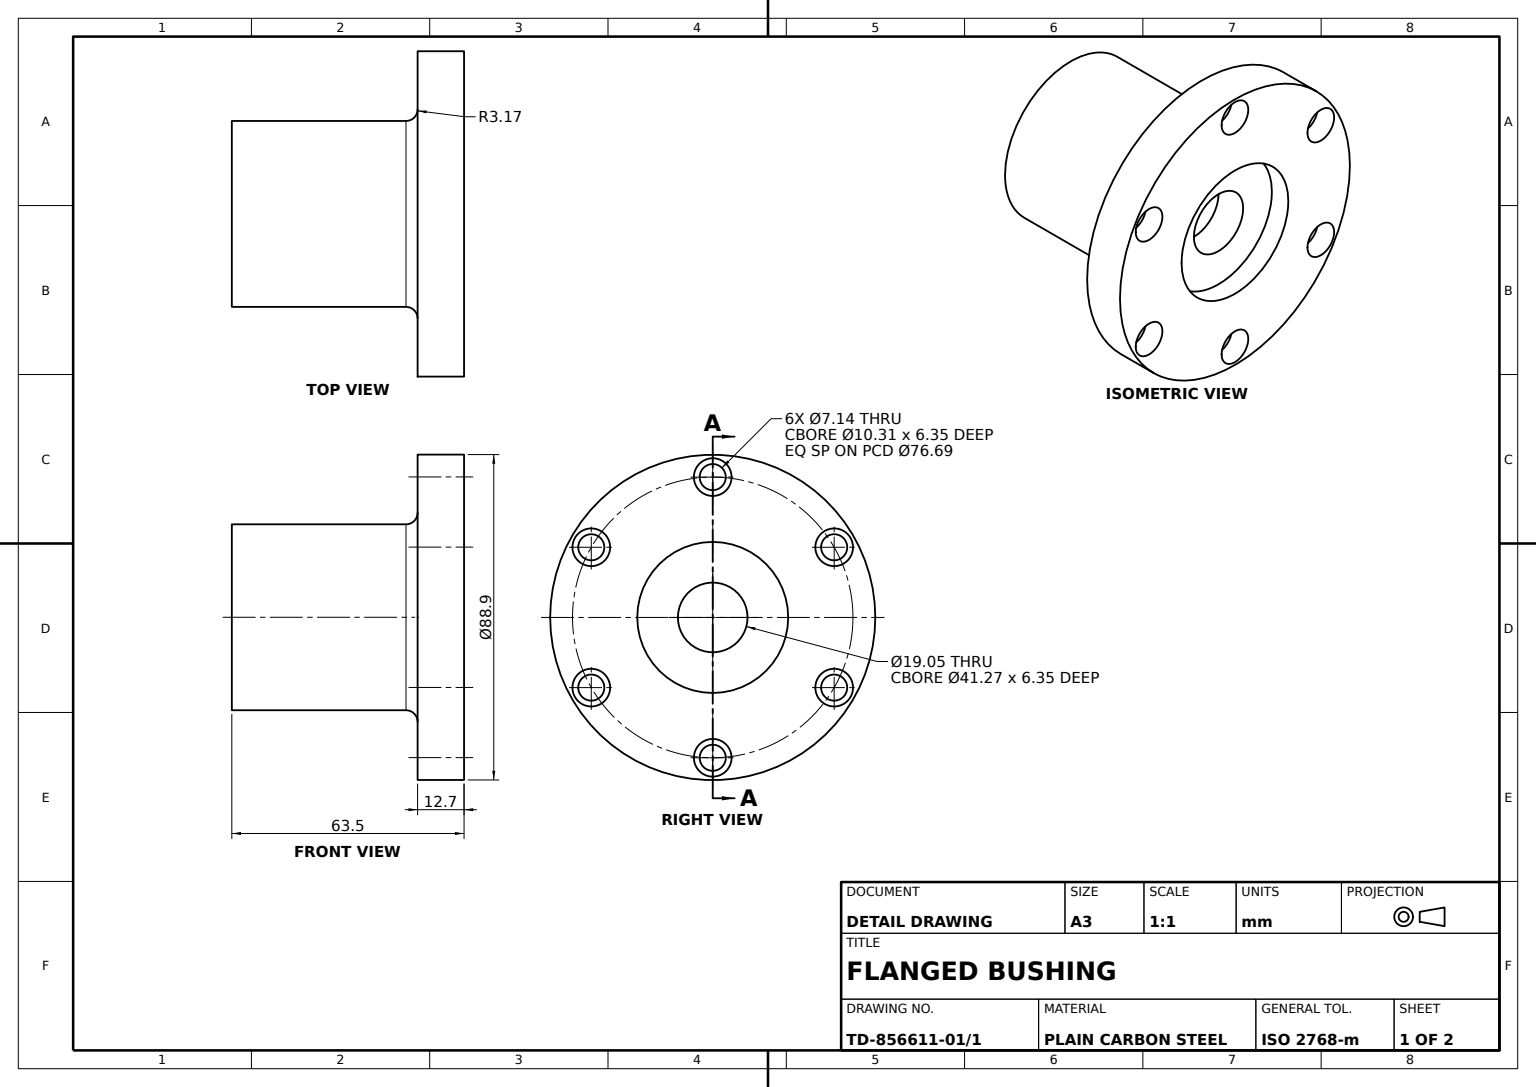
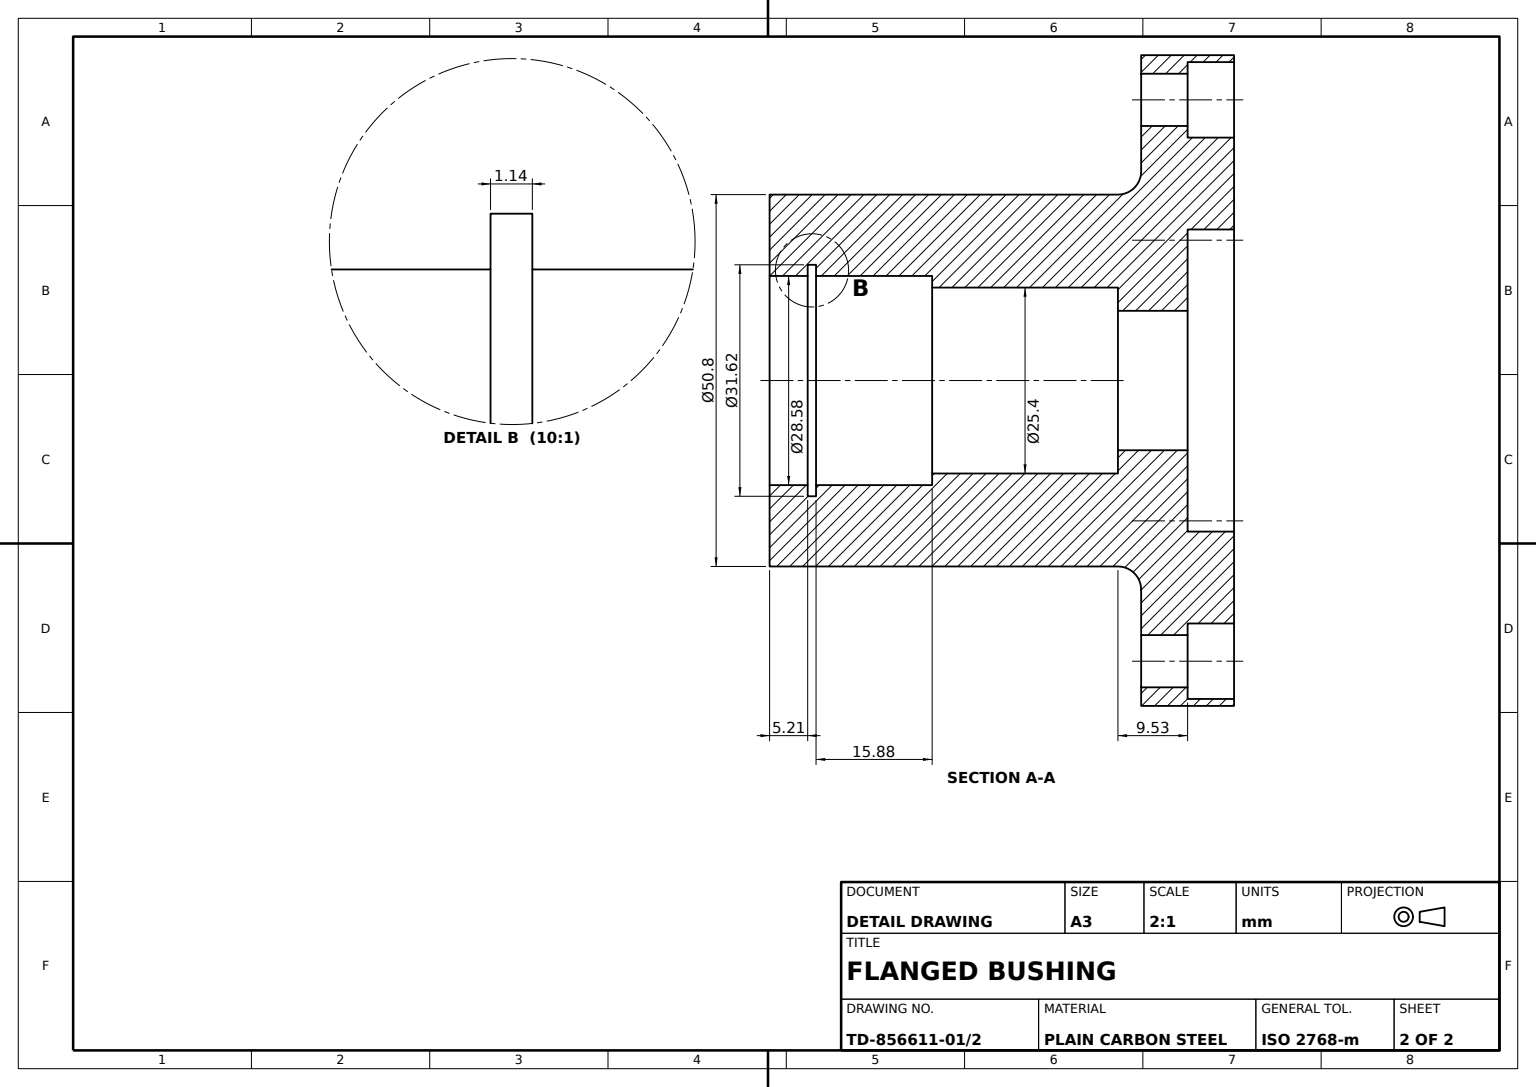
SolidWorks part; units mm, degrees
material "Plain Carbon Steel"
ref_plane "Front Plane" through (0, 0, 0) normal (0, 0, 1) x (1, 0, 0)
ref_plane "Top Plane" through (0, 0, 0) normal (0, 1, 0) x (1, 0, 0)
ref_plane "Right Plane" through (0, 0, 0) normal (1, 0, 0) x (0, 0, -1)
sketch "Flange Sketch" plane through (0, 0, 0) normal (0, 0, 1) x (1, 0, 0)
  circle A0 centre (0, 0) radius 44.45
  dimension "D1" = 88.9
extrude "Flange Ø3.5" add sketch "Flange Sketch" along normal blind 12.7
sketch "Hub Boss Sketch" plane through (0, 0, 12.7) normal (0, 0, 1) x (1, 0, 0)
  circle A0 centre (0, 0) radius 25.4
  dimension "D1" = 50.8
extrude "Hub Boss Ø2" add sketch "Hub Boss Sketch" along normal blind 50.8
sketch "Rear Recess Sketch" plane through (0, 0, 0) normal (0, 0, -1) x (-1, 0, 0)
  circle A0 centre (0, 0) radius 20.6375
  dimension "D1" = 41.275
extrude "Rear Recess Ø1.625" cut sketch "Rear Recess Sketch" against normal blind 6.35
sketch "Pilot Bore Sketch" plane through (0, 0, 6.35) normal (0, 0, -1) x (-1, 0, 0)
  circle A0 centre (0, 0) radius 9.525
  dimension "D1" = 19.05
extrude "Pilot Bore Ø0.75" cut sketch "Pilot Bore Sketch" against normal blind 9.525
sketch "Inner Bore Sketch" plane through (0, 0, 15.875) normal (0, 0, -1) x (-1, 0, 0)
  circle A0 centre (0, 0) radius 12.7
  dimension "D1" = 25.4
extrude "Inner Bore Ø1.0" cut sketch "Inner Bore Sketch" against normal blind 25.4
sketch "Bearing Bore Sketch" plane through (0, 0, 41.275) normal (0, 0, -1) x (-1, 0, 0)
  circle A0 centre (0, 0) radius 14.2875
  dimension "D1" = 28.575
extrude "Bearing Bore Ø1.125" cut sketch "Bearing Bore Sketch" against normal blind 15.875
sketch "Retaining Groove Sketch" plane through (0, 0, 57.15) normal (0, 0, -1) x (-1, 0, 0)
  circle A0 centre (0, 0) radius 15.8115
  dimension "D1" = 31.623
extrude "Retaining Ring Groove Ø1.245" cut sketch "Retaining Groove Sketch" against normal blind 1.143
sketch "Through Bore Sketch" plane through (0, 0, 58.293) normal (0, 0, -1) x (-1, 0, 0)
  circle A0 centre (0, 0) radius 14.2875
  dimension "D1" = 28.575
extrude "Through Bore Ø1.125" cut sketch "Through Bore Sketch" against normal through all
sketch "Bolt Counterbore Sketch" plane through (0, 0, 0) normal (0, 0, -1) x (-1, 0, 0)
  circle A1 centre (0, 38.3451) radius 5.1562
  circle A2 centre (33.2078, 19.1725) radius 5.1562
  circle A3 centre (33.2078, -19.1725) radius 5.1562
  circle A4 centre (0, -38.3451) radius 5.1562
  circle A5 centre (-33.2078, -19.1725) radius 5.1562
  circle A6 centre (-33.2078, 19.1725) radius 5.1562
  circle A7 centre (0, 0) radius 20.6375 construction
  point P15 (0, 0)
  dimension "D1" = 10.3124
  dimension "D3" = 33.2078
  dimension "D4" = 33.2078
  dimension "D5" = 19.1725
  dimension "D2" = 6
extrude "Bolt Counterbores 6xØ0.406" cut sketch "Bolt Counterbore Sketch" against normal blind 6.35
sketch "Bolt Hole Sketch" plane through (0, 0, 6.35) normal (0, 0, -1) x (-1, 0, 0)
  circle A0 centre (0, 38.3451) radius 3.5687
  circle A1 centre (33.2078, 19.1725) radius 3.5687
  circle A2 centre (33.2078, -19.1725) radius 3.5687
  circle A3 centre (0, -38.3451) radius 3.5687
  circle A4 centre (-33.2078, -19.1725) radius 3.5687
  circle A5 centre (-33.2078, 19.1725) radius 3.5687
  circle A6 centre (0, 38.3451) radius 5.1562 construction
  point P15 (0, 0)
  dimension "D1" = 7.1374
  dimension "D2" = 33.2078
extrude "Bolt Holes 6xØ0.281" cut sketch "Bolt Hole Sketch" against normal through all
fillet "Hub Root Fillet R0.125" radius 3.175 1 edges at (25.4, 0, 12.7)
